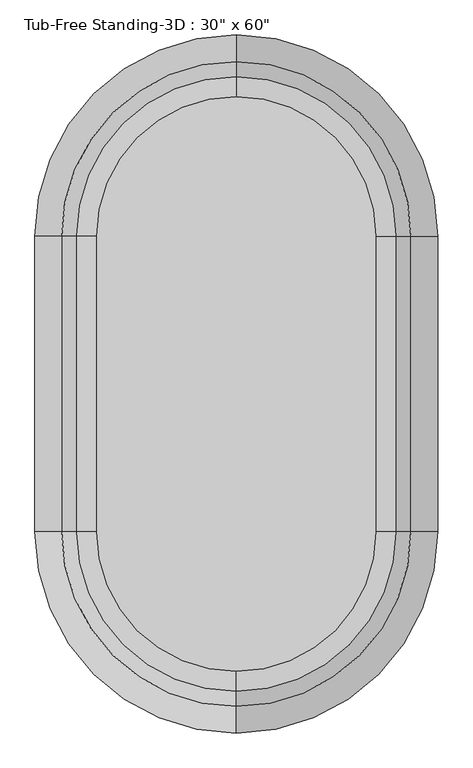
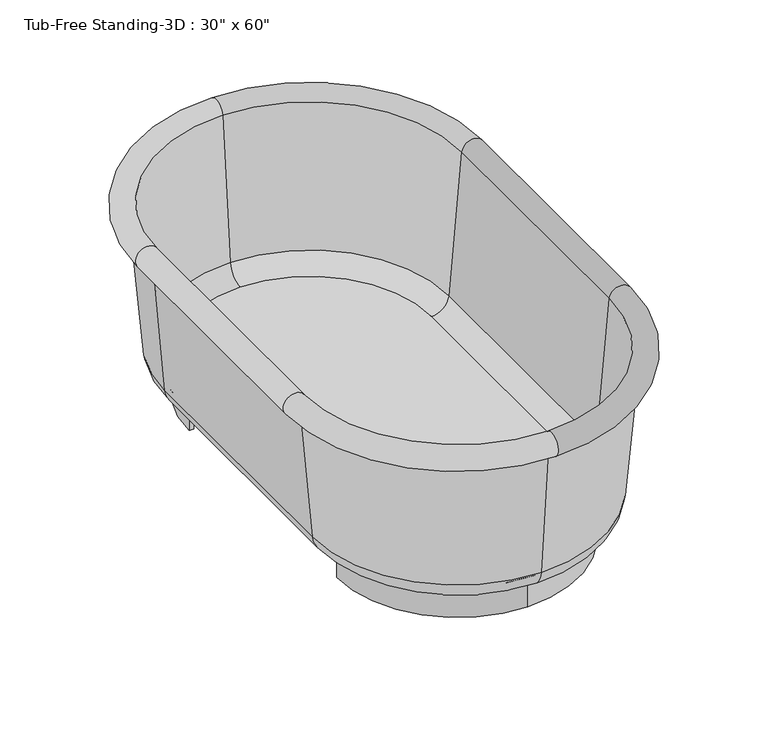
"""IFC4 building model written with IfcOpenShell, lengths in millimetres: flow terminal geometry."""

from ifc_helpers import new_model, si_unit, point, frame, frame_2d, origin, origin_with_axes, place, context, project, spatial, polyline, circle_curve, ellipse_curve, trimmed, segment, composite_curve, outline, extrude, source, transform, mapped, element, save
from ifc_brep_helpers import plane_surface, cylinder_surface, revolved_surface, advanced_brep


def flow_terminal_159a3241(model_context):
    return source(origin(), model_context, "Body", "SolidModel", [
        extrude(outline(composite_curve([segment(trimmed(circle_curve(frame_2d((0.0, 279.4)), 254.0), [point((0.0, 533.4))], [point((-254.0, 279.4))], True, "CARTESIAN"), True, "CONTINUOUS"), segment(polyline([(-254.0, 279.4), (-264.2824236, 279.4)]), True, "CONTINUOUS"), segment(trimmed(circle_curve(frame_2d((0.0, 279.4)), 264.2824236), [point((-264.2824236, 279.4))], [point((0.0, 543.6824236))], False, "CARTESIAN"), True, "CONTINUOUS"), segment(trimmed(circle_curve(frame_2d((0.0, 279.4)), 264.2824236), [point((0.0, 543.6824236))], [point((264.2824236, 279.4))], False, "CARTESIAN"), True, "CONTINUOUS"), segment(polyline([(264.2824236, 279.4), (254.0, 279.4)]), True, "CONTINUOUS"), segment(trimmed(circle_curve(frame_2d((0.0, 279.4)), 254.0), [point((254.0, 279.4))], [point((0.0, 533.4))], True, "CARTESIAN"), True, "CONTINUOUS")], self_intersect=False)), origin_with_axes(), (0.0, 0.0, 1.0), 63.5),
        extrude(outline(composite_curve([segment(trimmed(circle_curve(frame_2d((0.0, -279.4)), 264.2824236), [point((0.0, -543.6824236))], [point((-264.2824236, -279.4))], False, "CARTESIAN"), True, "CONTINUOUS"), segment(polyline([(-264.2824236, -279.4), (-254.0, -279.4)]), True, "CONTINUOUS"), segment(trimmed(circle_curve(frame_2d((0.0, -279.4)), 254.0), [point((-254.0, -279.4))], [point((0.0, -533.4))], True, "CARTESIAN"), True, "CONTINUOUS"), segment(trimmed(circle_curve(frame_2d((0.0, -279.4)), 254.0), [point((0.0, -533.4))], [point((254.0, -279.4))], True, "CARTESIAN"), True, "CONTINUOUS"), segment(polyline([(254.0, -279.4), (264.2824236, -279.4)]), True, "CONTINUOUS"), segment(trimmed(circle_curve(frame_2d((0.0, -279.4)), 264.2824236), [point((264.2824236, -279.4))], [point((0.0, -543.6824236))], False, "CARTESIAN"), True, "CONTINUOUS")], self_intersect=False)), origin_with_axes(), (0.0, 0.0, 1.0), 63.5),
        extrude(outline(composite_curve([segment(polyline([(-264.2824236, -279.4), (-264.2824236, 279.4)]), True, "CONTINUOUS"), segment(trimmed(circle_curve(frame_2d((0.0, 279.4)), 264.2824236), [point((-264.2824236, 279.4))], [point((0.0, 543.6824236))], False, "CARTESIAN"), True, "CONTINUOUS"), segment(trimmed(circle_curve(frame_2d((0.0, 279.4)), 264.2824236), [point((0.0, 543.6824236))], [point((264.2824236, 279.4))], False, "CARTESIAN"), True, "CONTINUOUS"), segment(polyline([(264.2824236, 279.4), (264.2824236, -279.4)]), True, "CONTINUOUS"), segment(trimmed(circle_curve(frame_2d((0.0, -279.4)), 264.2824236), [point((264.2824236, -279.4))], [point((0.0, -543.6824236))], False, "CARTESIAN"), True, "CONTINUOUS"), segment(trimmed(circle_curve(frame_2d((0.0, -279.4)), 264.2824236), [point((0.0, -543.6824236))], [point((-264.2824236, -279.4))], False, "CARTESIAN"), True, "CONTINUOUS")], self_intersect=False)), frame((0.0, 0.0, 63.5), z_axis=(0.0, 0.0, 1.0), x_axis=(1.0, 0.0, 0.0)), (0.0, 0.0, 1.0), 15.08125),
        advanced_brep(
        [(0.0, -622.3, 406.4), (342.9, -279.4, 406.4), (355.6, -279.4, 406.4), (0.0, -635.0, 406.4), (0.0, -596.5045038, 111.5561295), (317.1045038, -279.4, 111.5561295), (0.0, -543.6824236, 63.1536107), (264.2824236, -279.4, 63.1536107), (0.0, -543.6824236, 78.0774627), (264.2824236, -279.4, 78.0774627), (0.0, -581.6374416, 112.8568289), (302.2374416, -279.4, 112.8568289), (0.0, -609.8561556, 435.3982063), (330.4561556, -279.4, 435.3982063), (-342.9, -279.4, 406.4), (-355.6, -279.4, 406.4), (-317.1045038, -279.4, 111.5561295), (-264.2824236, -279.4, 63.1536107), (-264.2824236, -279.4, 78.0774627), (-302.2374416, -279.4, 112.8568289), (-330.4561556, -279.4, 435.3982063), (-355.6, 279.4, 406.4), (-342.9, 279.4, 406.4), (-317.1045038, 279.4, 111.5561295), (-264.2824236, 279.4, 63.1536107), (-264.2824236, 279.4, 78.0774627), (-302.2374416, 279.4, 112.8568289), (-330.4561556, 279.4, 435.3982063), (0.0, 622.3, 406.4), (0.0, 635.0, 406.4), (0.0, 596.5045038, 111.5561295), (0.0, 543.6824236, 63.1536107), (0.0, 543.6824236, 78.0774627), (0.0, 581.6374416, 112.8568289), (0.0, 609.8561556, 435.3982063), (342.9, 279.4, 406.4), (355.6, 279.4, 406.4), (317.1045038, 279.4, 111.5561295), (264.2824236, 279.4, 63.1536107), (264.2824236, 279.4, 78.0774627), (302.2374416, 279.4, 112.8568289), (330.4561556, 279.4, 435.3982063)],
        [
            (0, 1, circle_curve(frame((0.0, -279.4, 406.4), z_axis=(0.0, 0.0, 1.0), x_axis=(1.0, 0.0, 0.0)), 342.9)),
            (1, 2),
            (2, 3, circle_curve(frame((0.0, -279.4, 406.4), z_axis=(0.0, 0.0, -1.0), x_axis=(1.0, 0.0, 0.0)), 355.6)),
            (3, 0),
            (4, 5, circle_curve(frame((0.0, -279.4, 111.5561295), z_axis=(0.0, 0.0, 1.0), x_axis=(1.0, 0.0, 0.0)), 317.1045038)),
            (5, 1),
            (0, 4),
            (6, 7, circle_curve(frame((0.0, -279.4, 63.1536107), z_axis=(0.0, 0.0, 1.0), x_axis=(1.0, 0.0, 0.0)), 264.2824236)),
            (7, 5, circle_curve(frame((264.2824236, -279.4, 116.1774627), z_axis=(0.0, -1.0, 0.0), x_axis=(1.0, 0.0, 0.0)), 53.023852)),
            (4, 6, circle_curve(frame((0.0, -543.6824236, 116.1774627), z_axis=(1.0, 0.0, 0.0), x_axis=(0.0, -1.0, 0.0)), 53.023852)),
            (8, 9, circle_curve(frame((0.0, -279.4, 78.0774627), z_axis=(0.0, 0.0, 1.0), x_axis=(1.0, 0.0, 0.0)), 264.2824236)),
            (9, 7),
            (6, 8),
            (10, 11, circle_curve(frame((0.0, -279.4, 112.8568289), z_axis=(0.0, 0.0, 1.0), x_axis=(1.0, 0.0, 0.0)), 302.2374416)),
            (11, 9, circle_curve(frame((264.2824236, -279.4, 116.1774627), z_axis=(0.0, 1.0, 0.0), x_axis=(1.0, 0.0, 0.0)), 38.1)),
            (8, 10, circle_curve(frame((0.0, -543.6824236, 116.1774627), z_axis=(-1.0, 0.0, 0.0), x_axis=(0.0, -1.0, 0.0)), 38.1)),
            (12, 13, circle_curve(frame((0.0, -279.4, 435.3982063), z_axis=(0.0, 0.0, 1.0), x_axis=(1.0, 0.0, 0.0)), 330.4561556)),
            (13, 11),
            (10, 12),
            (2, 13, circle_curve(frame((355.6, -279.4, 431.8), z_axis=(0.0, -1.0, 0.0), x_axis=(1.0, 0.0, 0.0)), 25.4)),
            (12, 3, circle_curve(frame((0.0, -635.0, 431.8), z_axis=(1.0, 0.0, 0.0), x_axis=(0.0, -1.0, 0.0)), 25.4)),
            (14, 0, circle_curve(frame((0.0, -279.4, 406.4), z_axis=(0.0, 0.0, 1.0), x_axis=(0.0, -1.0, 0.0)), 342.9)),
            (3, 15, circle_curve(frame((0.0, -279.4, 406.4), z_axis=(0.0, 0.0, -1.0), x_axis=(0.0, -1.0, 0.0)), 355.6)),
            (15, 14),
            (16, 4, circle_curve(frame((0.0, -279.4, 111.5561295), z_axis=(0.0, 0.0, 1.0), x_axis=(0.0, -1.0, 0.0)), 317.1045038)),
            (14, 16),
            (17, 6, circle_curve(frame((0.0, -279.4, 63.1536107), z_axis=(0.0, 0.0, 1.0), x_axis=(0.0, -1.0, 0.0)), 264.2824236)),
            (16, 17, circle_curve(frame((-264.2824236, -279.4, 116.1774627), z_axis=(0.0, -1.0, 0.0), x_axis=(-1.0, 0.0, 0.0)), 53.023852)),
            (18, 8, circle_curve(frame((0.0, -279.4, 78.0774627), z_axis=(0.0, 0.0, 1.0), x_axis=(0.0, -1.0, 0.0)), 264.2824236)),
            (17, 18),
            (19, 10, circle_curve(frame((0.0, -279.4, 112.8568289), z_axis=(0.0, 0.0, 1.0), x_axis=(0.0, -1.0, 0.0)), 302.2374416)),
            (18, 19, circle_curve(frame((-264.2824236, -279.4, 116.1774627), z_axis=(0.0, 1.0, 0.0), x_axis=(-1.0, 0.0, 0.0)), 38.1)),
            (20, 12, circle_curve(frame((0.0, -279.4, 435.3982063), z_axis=(0.0, 0.0, 1.0), x_axis=(0.0, -1.0, 0.0)), 330.4561556)),
            (19, 20),
            (20, 15, circle_curve(frame((-355.6, -279.4, 431.8), z_axis=(0.0, -1.0, 0.0), x_axis=(-1.0, 0.0, 0.0)), 25.4)),
            (15, 21),
            (21, 22),
            (22, 14),
            (22, 23),
            (23, 16),
            (23, 24, circle_curve(frame((-264.2824236, 279.4, 116.1774627), z_axis=(0.0, -1.0, 0.0), x_axis=(-1.0, 0.0, 0.0)), 53.023852)),
            (24, 17),
            (24, 25),
            (25, 18),
            (25, 26, circle_curve(frame((-264.2824236, 279.4, 116.1774627), z_axis=(0.0, 1.0, 0.0), x_axis=(-1.0, 0.0, 0.0)), 38.1)),
            (26, 19),
            (26, 27),
            (27, 20),
            (27, 21, circle_curve(frame((-355.6, 279.4, 431.8), z_axis=(0.0, -1.0, 0.0), x_axis=(-1.0, 0.0, 0.0)), 25.4)),
            (28, 22, circle_curve(frame((0.0, 279.4, 406.4), z_axis=(0.0, 0.0, 1.0), x_axis=(-1.0, 0.0, 0.0)), 342.9)),
            (21, 29, circle_curve(frame((0.0, 279.4, 406.4), z_axis=(0.0, 0.0, -1.0), x_axis=(-1.0, 0.0, 0.0)), 355.6)),
            (29, 28),
            (30, 23, circle_curve(frame((0.0, 279.4, 111.5561295), z_axis=(0.0, 0.0, 1.0), x_axis=(-1.0, 0.0, 0.0)), 317.1045038)),
            (28, 30),
            (31, 24, circle_curve(frame((0.0, 279.4, 63.1536107), z_axis=(0.0, 0.0, 1.0), x_axis=(-1.0, 0.0, 0.0)), 264.2824236)),
            (30, 31, circle_curve(frame((0.0, 543.6824236, 116.1774627), z_axis=(-1.0, 0.0, 0.0), x_axis=(0.0, 1.0, 0.0)), 53.023852)),
            (32, 25, circle_curve(frame((0.0, 279.4, 78.0774627), z_axis=(0.0, 0.0, 1.0), x_axis=(-1.0, 0.0, 0.0)), 264.2824236)),
            (31, 32),
            (33, 26, circle_curve(frame((0.0, 279.4, 112.8568289), z_axis=(0.0, 0.0, 1.0), x_axis=(-1.0, 0.0, 0.0)), 302.2374416)),
            (32, 33, circle_curve(frame((0.0, 543.6824236, 116.1774627), z_axis=(1.0, 0.0, 0.0), x_axis=(0.0, 1.0, 0.0)), 38.1)),
            (34, 27, circle_curve(frame((0.0, 279.4, 435.3982063), z_axis=(0.0, 0.0, 1.0), x_axis=(-1.0, 0.0, 0.0)), 330.4561556)),
            (33, 34),
            (34, 29, circle_curve(frame((0.0, 635.0, 431.8), z_axis=(-1.0, 0.0, 0.0), x_axis=(0.0, 1.0, 0.0)), 25.4)),
            (35, 28, circle_curve(frame((0.0, 279.4, 406.4), z_axis=(0.0, 0.0, 1.0), x_axis=(0.0, 1.0, 0.0)), 342.9)),
            (29, 36, circle_curve(frame((0.0, 279.4, 406.4), z_axis=(0.0, 0.0, -1.0), x_axis=(0.0, 1.0, 0.0)), 355.6)),
            (36, 35),
            (37, 30, circle_curve(frame((0.0, 279.4, 111.5561295), z_axis=(0.0, 0.0, 1.0), x_axis=(0.0, 1.0, 0.0)), 317.1045038)),
            (35, 37),
            (38, 31, circle_curve(frame((0.0, 279.4, 63.1536107), z_axis=(0.0, 0.0, 1.0), x_axis=(0.0, 1.0, 0.0)), 264.2824236)),
            (37, 38, circle_curve(frame((264.2824236, 279.4, 116.1774627), z_axis=(0.0, 1.0, 0.0), x_axis=(1.0, 0.0, 0.0)), 53.023852)),
            (39, 32, circle_curve(frame((0.0, 279.4, 78.0774627), z_axis=(0.0, 0.0, 1.0), x_axis=(0.0, 1.0, 0.0)), 264.2824236)),
            (38, 39),
            (40, 33, circle_curve(frame((0.0, 279.4, 112.8568289), z_axis=(0.0, 0.0, 1.0), x_axis=(0.0, 1.0, 0.0)), 302.2374416)),
            (39, 40, circle_curve(frame((264.2824236, 279.4, 116.1774627), z_axis=(0.0, -1.0, 0.0), x_axis=(1.0, 0.0, 0.0)), 38.1)),
            (41, 34, circle_curve(frame((0.0, 279.4, 435.3982063), z_axis=(0.0, 0.0, 1.0), x_axis=(0.0, 1.0, 0.0)), 330.4561556)),
            (40, 41),
            (41, 36, circle_curve(frame((355.6, 279.4, 431.8), z_axis=(0.0, 1.0, 0.0), x_axis=(1.0, 0.0, 0.0)), 25.4)),
            (36, 2),
            (1, 35),
            (5, 37),
            (7, 38),
            (9, 39),
            (11, 40),
            (13, 41),
        ],
        [
            plane_surface(frame((0.0, -279.4, 406.4), z_axis=(0.0, 0.0, -1.0), x_axis=(1.0, 0.0, 0.0))),
            revolved_surface(polyline([(342.9, -279.4, 406.4), (317.1045038, -279.4, 111.5561295)]), (0.0, -279.4, 431.8), (0.0, 0.0, -1.0)),
            revolved_surface(trimmed(ellipse_curve(frame((264.2824236, -279.4, 116.1774627), z_axis=(0.0, 1.0, 0.0), x_axis=(1.0, 0.0, 0.0)), 53.023852, 53.023852), [point((317.1045038, -279.4, 111.5561295))], [point((264.2824236, -279.4, 63.1536107))], True, "CARTESIAN"), (0.0, -279.4, 431.8), (0.0, 0.0, -1.0)),
            revolved_surface(polyline([(264.2824236, -279.4, 63.1536107), (264.2824236, -279.4, 78.07746270000001)]), (0.0, -279.4, 431.8), (0.0, 0.0, -1.0)),
            revolved_surface(trimmed(ellipse_curve(frame((264.2824236, -279.4, 116.1774627), z_axis=(0.0, -1.0, 0.0), x_axis=(1.0, 0.0, 0.0)), 38.1, 38.1), [point((264.2824236, -279.4, 78.0774627))], [point((302.2374416, -279.4, 112.8568289))], True, "CARTESIAN"), (0.0, -279.4, 431.8), (0.0, 0.0, -1.0)),
            revolved_surface(polyline([(302.2374416, -279.4, 112.8568289), (330.4561556, -279.4, 435.3982063)]), (0.0, -279.4, 431.8), (0.0, 0.0, -1.0)),
            revolved_surface(trimmed(ellipse_curve(frame((355.6, -279.4, 431.8), z_axis=(0.0, 1.0, 0.0), x_axis=(1.0, 0.0, 0.0)), 25.4, 25.4), [point((330.4561556, -279.4, 435.3982063))], [point((355.6, -279.4, 406.4))], True, "CARTESIAN"), (0.0, -279.4, 431.8), (0.0, 0.0, -1.0)),
            plane_surface(frame((0.0, -279.4, 406.4), z_axis=(0.0, 0.0, -1.0), x_axis=(0.0, -1.0, 0.0))),
            revolved_surface(polyline([(0.0, -622.3, 406.4), (0.0, -596.5045038, 111.5561295)]), (0.0, -279.4, 431.8), (0.0, 0.0, -1.0)),
            revolved_surface(trimmed(ellipse_curve(frame((0.0, -543.6824236, 116.1774627), z_axis=(1.0, 0.0, 0.0), x_axis=(0.0, -1.0, 0.0)), 53.023852, 53.023852), [point((0.0, -596.5045038, 111.5561295))], [point((0.0, -543.6824236, 63.1536107))], True, "CARTESIAN"), (0.0, -279.4, 431.8), (0.0, 0.0, -1.0)),
            revolved_surface(polyline([(0.0, -543.6824236, 63.1536107), (0.0, -543.6824236, 78.07746270000001)]), (0.0, -279.4, 431.8), (0.0, 0.0, -1.0)),
            revolved_surface(trimmed(ellipse_curve(frame((0.0, -543.6824236, 116.1774627), z_axis=(-1.0, 0.0, 0.0), x_axis=(0.0, -1.0, 0.0)), 38.1, 38.1), [point((0.0, -543.6824236, 78.0774627))], [point((0.0, -581.6374416, 112.8568289))], True, "CARTESIAN"), (0.0, -279.4, 431.8), (0.0, 0.0, -1.0)),
            revolved_surface(polyline([(0.0, -581.6374416, 112.8568289), (0.0, -609.8561556, 435.3982063)]), (0.0, -279.4, 431.8), (0.0, 0.0, -1.0)),
            revolved_surface(trimmed(ellipse_curve(frame((0.0, -635.0, 431.8), z_axis=(1.0, 0.0, 0.0), x_axis=(0.0, -1.0, 0.0)), 25.4, 25.4), [point((0.0, -609.8561556, 435.3982063))], [point((0.0, -635.0, 406.4))], True, "CARTESIAN"), (0.0, -279.4, 431.8), (0.0, 0.0, -1.0)),
            plane_surface(frame((-355.6, -279.4, 406.4), z_axis=(0.0, 0.0, -1.0), x_axis=(0.0, 1.0, 0.0))),
            plane_surface(frame((-342.9, -279.4, 406.4), z_axis=(-0.9961946980917455, 0.0, -0.08715574274765871), x_axis=(0.0, 1.0, 0.0))),
            cylinder_surface(frame((-264.2824236, -279.4, 116.1774627), z_axis=(0.0, -1.0, 0.0), x_axis=(-1.0, 0.0, 0.0)), 53.023852),
            plane_surface(frame((-264.2824236, -279.4, 63.1536107), z_axis=(1.0, 0.0, 0.0), x_axis=(0.0, 1.0, 0.0))),
            revolved_surface(polyline([(-302.38242360000004, 279.4, 116.1774627), (-302.38242360000004, -279.4, 116.1774627)]), (-264.2824236, -279.4, 116.1774627), (0.0, 1.0, 0.0)),
            plane_surface(frame((-302.2374416, -279.4, 112.8568289), z_axis=(0.9961946980917458, 0.0, 0.08715574274765651), x_axis=(0.0, 1.0, 0.0))),
            cylinder_surface(frame((-355.6, -279.4, 431.8), z_axis=(0.0, -1.0, 0.0), x_axis=(-1.0, 0.0, 0.0)), 25.4),
            plane_surface(frame((0.0, 279.4, 406.4), z_axis=(0.0, 0.0, -1.0), x_axis=(-1.0, 0.0, 0.0))),
            revolved_surface(polyline([(-342.9, 279.4, 406.4), (-317.1045038, 279.4, 111.5561295)]), (0.0, 279.4, 431.8), (0.0, 0.0, -1.0)),
            revolved_surface(trimmed(ellipse_curve(frame((-264.2824236, 279.4, 116.1774627), z_axis=(0.0, -1.0, 0.0), x_axis=(-1.0, 0.0, 0.0)), 53.023852, 53.023852), [point((-317.1045038, 279.4, 111.5561295))], [point((-264.2824236, 279.4, 63.1536107))], True, "CARTESIAN"), (0.0, 279.4, 431.8), (0.0, 0.0, -1.0)),
            revolved_surface(polyline([(-264.2824236, 279.4, 63.1536107), (-264.2824236, 279.4, 78.07746270000001)]), (0.0, 279.4, 431.8), (0.0, 0.0, -1.0)),
            revolved_surface(trimmed(ellipse_curve(frame((-264.2824236, 279.4, 116.1774627), z_axis=(0.0, 1.0, 0.0), x_axis=(-1.0, 0.0, 0.0)), 38.1, 38.1), [point((-264.2824236, 279.4, 78.0774627))], [point((-302.2374416, 279.4, 112.8568289))], True, "CARTESIAN"), (0.0, 279.4, 431.8), (0.0, 0.0, -1.0)),
            revolved_surface(polyline([(-302.2374416, 279.4, 112.8568289), (-330.4561556, 279.4, 435.3982063)]), (0.0, 279.4, 431.8), (0.0, 0.0, -1.0)),
            revolved_surface(trimmed(ellipse_curve(frame((-355.6, 279.4, 431.8), z_axis=(0.0, -1.0, 0.0), x_axis=(-1.0, 0.0, 0.0)), 25.4, 25.4), [point((-330.4561556, 279.4, 435.3982063))], [point((-355.6, 279.4, 406.4))], True, "CARTESIAN"), (0.0, 279.4, 431.8), (0.0, 0.0, -1.0)),
            plane_surface(frame((0.0, 279.4, 406.4), z_axis=(0.0, 0.0, -1.0), x_axis=(0.0, 1.0, 0.0))),
            revolved_surface(polyline([(0.0, 622.3, 406.4), (0.0, 596.5045038, 111.5561295)]), (0.0, 279.4, 431.8), (0.0, 0.0, -1.0)),
            revolved_surface(trimmed(ellipse_curve(frame((0.0, 543.6824236, 116.1774627), z_axis=(-1.0, 0.0, 0.0), x_axis=(0.0, 1.0, 0.0)), 53.023852, 53.023852), [point((0.0, 596.5045038, 111.5561295))], [point((0.0, 543.6824236, 63.1536107))], True, "CARTESIAN"), (0.0, 279.4, 431.8), (0.0, 0.0, -1.0)),
            revolved_surface(polyline([(0.0, 543.6824236, 63.1536107), (0.0, 543.6824236, 78.07746270000001)]), (0.0, 279.4, 431.8), (0.0, 0.0, -1.0)),
            revolved_surface(trimmed(ellipse_curve(frame((0.0, 543.6824236, 116.1774627), z_axis=(1.0, 0.0, 0.0), x_axis=(0.0, 1.0, 0.0)), 38.1, 38.1), [point((0.0, 543.6824236, 78.0774627))], [point((0.0, 581.6374416, 112.8568289))], True, "CARTESIAN"), (0.0, 279.4, 431.8), (0.0, 0.0, -1.0)),
            revolved_surface(polyline([(0.0, 581.6374416, 112.8568289), (0.0, 609.8561556, 435.3982063)]), (0.0, 279.4, 431.8), (0.0, 0.0, -1.0)),
            revolved_surface(trimmed(ellipse_curve(frame((0.0, 635.0, 431.8), z_axis=(-1.0, 0.0, 0.0), x_axis=(0.0, 1.0, 0.0)), 25.4, 25.4), [point((0.0, 609.8561556, 435.3982063))], [point((0.0, 635.0, 406.4))], True, "CARTESIAN"), (0.0, 279.4, 431.8), (0.0, 0.0, -1.0)),
            plane_surface(frame((355.6, 279.4, 406.4), z_axis=(0.0, 0.0, -1.0), x_axis=(0.0, -1.0, 0.0))),
            plane_surface(frame((342.9, 279.4, 406.4), z_axis=(0.9961946980917455, 0.0, -0.08715574274765871), x_axis=(0.0, -1.0, 0.0))),
            cylinder_surface(frame((264.2824236, 279.4, 116.1774627), z_axis=(0.0, 1.0, 0.0), x_axis=(1.0, 0.0, 0.0)), 53.023852),
            plane_surface(frame((264.2824236, 279.4, 63.1536107), z_axis=(-1.0, 0.0, 0.0), x_axis=(0.0, -1.0, 0.0))),
            revolved_surface(polyline([(302.38242360000004, -279.4, 116.1774627), (302.38242360000004, 279.4, 116.1774627)]), (264.2824236, 279.4, 116.1774627), (0.0, -1.0, 0.0)),
            plane_surface(frame((302.2374416, 279.4, 112.8568289), z_axis=(-0.9961946980917458, 0.0, 0.08715574274765651), x_axis=(0.0, -1.0, 0.0))),
            cylinder_surface(frame((355.6, 279.4, 431.8), z_axis=(0.0, 1.0, 0.0), x_axis=(1.0, 0.0, 0.0)), 25.4),
        ],
        [
            (0, [[1, 2, 3, 4]]),
            (1, [[5, 6, -1, 7]]),
            (2, [[8, 9, -5, 10]]),
            (3, [[11, 12, -8, 13]]),
            (4, [[14, 15, -11, 16]]),
            (5, [[17, 18, -14, 19]]),
            (6, [[-3, 20, -17, 21]]),
            (7, [[22, -4, 23, 24]]),
            (8, [[25, -7, -22, 26]]),
            (9, [[27, -10, -25, 28]]),
            (10, [[29, -13, -27, 30]]),
            (11, [[31, -16, -29, 32]]),
            (12, [[33, -19, -31, 34]]),
            (13, [[-23, -21, -33, 35]]),
            (14, [[-24, 36, 37, 38]]),
            (15, [[-26, -38, 39, 40]]),
            (16, [[-28, -40, 41, 42]]),
            (17, [[-30, -42, 43, 44]]),
            (18, [[-32, -44, 45, 46]]),
            (19, [[-34, -46, 47, 48]]),
            (20, [[-35, -48, 49, -36]]),
            (21, [[50, -37, 51, 52]]),
            (22, [[53, -39, -50, 54]]),
            (23, [[55, -41, -53, 56]]),
            (24, [[57, -43, -55, 58]]),
            (25, [[59, -45, -57, 60]]),
            (26, [[61, -47, -59, 62]]),
            (27, [[-51, -49, -61, 63]]),
            (28, [[64, -52, 65, 66]]),
            (29, [[67, -54, -64, 68]]),
            (30, [[69, -56, -67, 70]]),
            (31, [[71, -58, -69, 72]]),
            (32, [[73, -60, -71, 74]]),
            (33, [[75, -62, -73, 76]]),
            (34, [[-65, -63, -75, 77]]),
            (35, [[-66, 78, -2, 79]]),
            (36, [[-68, -79, -6, 80]]),
            (37, [[-70, -80, -9, 81]]),
            (38, [[-72, -81, -12, 82]]),
            (39, [[-74, -82, -15, 83]]),
            (40, [[-76, -83, -18, 84]]),
            (41, [[-77, -84, -20, -78]]),
        ],
    ),
    ])


if __name__ == "__main__":
    model = new_model("IFC4")
    model_context = context("Model", 3, world=origin())
    ifc_project = project(units=[si_unit("LENGTHUNIT", "METRE", prefix="MILLI")], contexts=[model_context])
    site = spatial("IfcSite", under=ifc_project)
    building = spatial("IfcBuilding", under=site)
    placement = place(None, origin())
    flow_terminal_shape = flow_terminal_159a3241(model_context)
    element("IfcFlowTerminal", 1, ObjectType="Tub-Free Standing-3D : 30\" x 60\"", at=placement, inside=building, context=model_context, shape_type="MappedRepresentation", body=[
        mapped(flow_terminal_shape, transform((0.0, 0.0, 0.0), x_axis=(1.0, 0.0, 0.0), y_axis=(0.0, 1.0, 0.0), z_axis=(0.0, 0.0, 1.0))),
    ])
    save(model, "model.ifc")

# Revit data of these elements
# Type "Tub-Free Standing-3D : 30\" x 60\""
#   Assembly Code = "D2010110"
#   Height = 1' - 6"
#   Length = 4' - 4"
#   Width = 2' - 6"
#   Tub Material = Porcelain, Ivory
#   Default Elevation = 0
# Element 1 (IfcFlowTerminal, "Tub-Free Standing-3D : 30\" x 60\"")
#   Materials on its faces: "Porcelain, Ivory"
# Materials
#   "Porcelain, Ivory": class "Ceramic", colour RGB 247 247 239, transparency 0, Description = "Porcelain, ivory", Cost = 0
